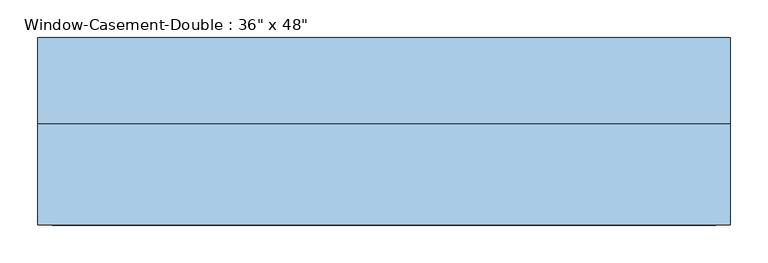
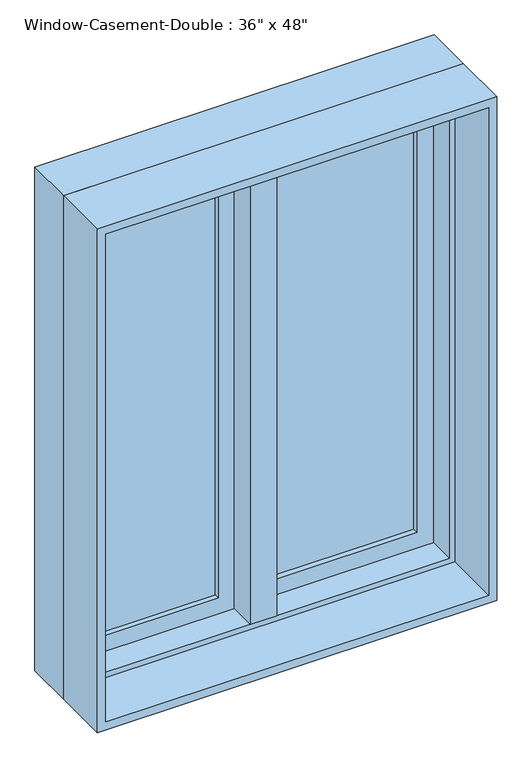
"""IFC4 building model written with IfcOpenShell, lengths in millimetres: window geometry."""

from ifc_helpers import new_model, si_unit, frame, origin, place, context, project, spatial, polyline, outline, extrude, faceted_brep, source, transform, mapped, element, save


def window_d341e8ac(model_context):
    return source(origin(), model_context, "Body", "SolidModel", [
        faceted_brep([(9.525, 133.35, 2120.9), (-9.525, 133.35, 2120.9), (-9.525, 82.55, 2120.9), (9.525, 82.55, 2120.9), (9.525, 133.35, 927.1), (9.525, 82.55, 927.1), (-9.525, 82.55, 927.1), (-9.525, 133.35, 927.1), (-9.525, 82.55, 946.15), (-9.525, 82.55, 2101.85), (-30.1625, 82.55, 946.15), (-30.1625, 82.55, 2101.85), (-30.1625, 19.05, 946.15), (-30.1625, 19.05, 2101.85), (30.1625, 19.05, 946.15), (30.1625, 19.05, 2101.85), (30.1625, 82.55, 946.15), (30.1625, 82.55, 2101.85), (9.525, 82.55, 946.15), (9.525, 82.55, 2101.85)], [[[0, 1, 2, 3]], [[4, 5, 6, 7]], [[1, 0, 4, 7]], [[2, 1, 7, 6, 8, 9]], [[9, 8, 10, 11]], [[11, 10, 12, 13]], [[13, 12, 14, 15]], [[15, 14, 16, 17]], [[17, 16, 18, 19]], [[0, 3, 19, 18, 5, 4]], [[18, 8, 6, 5]], [[9, 19, 3, 2]], [[8, 18, 16, 14, 12, 10]], [[19, 9, 11, 13, 15, 17]]]),
        extrude(outline(polyline([(-66.675, 114.3), (-66.675, 107.95), (-387.35, 107.95), (-387.35, 114.3), (-66.675, 114.3)])), frame((0.0, 0.0, 984.25), z_axis=(0.0, 0.0, 1.0), x_axis=(1.0, 0.0, 0.0)), (0.0, 0.0, 1.0), 1079.5),
        extrude(outline(polyline([(-387.35, 95.25), (-387.35, 101.6), (-66.675, 101.6), (-66.675, 95.25), (-387.35, 95.25)])), frame((0.0, 0.0, 984.25), z_axis=(0.0, 0.0, 1.0), x_axis=(1.0, 0.0, 0.0)), (0.0, 0.0, 1.0), 1079.5),
        extrude(outline(polyline([(387.35, 114.3), (387.35, 107.95), (66.675, 107.95), (66.675, 114.3), (387.35, 114.3)])), frame((0.0, 0.0, 984.25), z_axis=(0.0, 0.0, 1.0), x_axis=(1.0, 0.0, 0.0)), (0.0, 0.0, 1.0), 1079.5),
        extrude(outline(polyline([(66.675, 95.25), (66.675, 101.6), (387.35, 101.6), (387.35, 95.25), (66.675, 95.25)])), frame((0.0, 0.0, 984.25), z_axis=(0.0, 0.0, 1.0), x_axis=(1.0, 0.0, 0.0)), (0.0, 0.0, 1.0), 1079.5),
        extrude(outline(polyline([(2120.9, -444.5), (927.1, -444.5), (927.1, -9.525), (2120.9, -9.525), (2120.9, -444.5)]), holes=[polyline([(2063.75, -66.675), (984.25, -66.675), (984.25, -387.35), (2063.75, -387.35), (2063.75, -66.675)])]), frame((0.0, 82.55, 0.0), z_axis=(0.0, 1.0, 0.0), x_axis=(0.0, 0.0, 1.0)), (0.0, 0.0, 1.0), 44.45),
        extrude(outline(polyline([(927.1, 444.5), (2120.9, 444.5), (2120.9, 9.525), (927.1, 9.525), (927.1, 444.5)]), holes=[polyline([(984.25, 66.675), (2063.75, 66.675), (2063.75, 387.35), (984.25, 387.35), (984.25, 66.675)])]), frame((0.0, 82.55, 0.0), z_axis=(0.0, 1.0, 0.0), x_axis=(0.0, 0.0, 1.0)), (0.0, 0.0, 1.0), 44.45),
        extrude(outline(polyline([(2133.6, -457.2), (914.4, -457.2), (914.4, 457.2), (2133.6, 457.2), (2133.6, -457.2)]), holes=[polyline([(2114.55, 438.15), (933.45, 438.15), (933.45, -438.15), (2114.55, -438.15), (2114.55, 438.15)])]), frame((0.0, -114.3, 0.0), z_axis=(0.0, 1.0, 0.0), x_axis=(0.0, 0.0, 1.0)), (0.0, 0.0, 1.0), 133.35),
        faceted_brep([(425.45, 82.55, 2101.85), (425.45, 19.05, 2101.85), (-425.45, 19.05, 2101.85), (-425.45, 82.55, 2101.85), (444.5, 133.35, 2120.9), (444.5, 82.55, 2120.9), (-444.5, 82.55, 2120.9), (-444.5, 133.35, 2120.9), (457.2, 19.05, 2133.6), (457.2, 133.35, 2133.6), (-457.2, 133.35, 2133.6), (-457.2, 19.05, 2133.6), (-425.45, 19.05, 946.15), (-425.45, 82.55, 946.15), (-444.5, 82.55, 927.1), (-444.5, 133.35, 927.1), (-457.2, 133.35, 914.4), (-457.2, 19.05, 914.4), (425.45, 19.05, 946.15), (425.45, 82.55, 946.15), (444.5, 82.55, 927.1), (444.5, 133.35, 927.1), (457.2, 133.35, 914.4), (457.2, 19.05, 914.4)], [[[0, 1, 2, 3]], [[4, 5, 6, 7]], [[8, 9, 10, 11]], [[3, 2, 12, 13]], [[7, 6, 14, 15]], [[11, 10, 16, 17]], [[13, 12, 18, 19]], [[15, 14, 20, 21]], [[17, 16, 22, 23]], [[11, 17, 23, 8], [1, 18, 12, 2]], [[19, 18, 1, 0]], [[5, 20, 14, 6], [3, 13, 19, 0]], [[21, 20, 5, 4]], [[23, 22, 9, 8]], [[9, 22, 16, 10], [7, 15, 21, 4]]]),
    ])


if __name__ == "__main__":
    model = new_model("IFC4")
    model_context = context("Model", 3, world=origin())
    ifc_project = project(units=[si_unit("LENGTHUNIT", "METRE", prefix="MILLI")], contexts=[model_context])
    site = spatial("IfcSite", under=ifc_project)
    building = spatial("IfcBuilding", under=site)
    placement = place(None, origin())
    window_shape = window_d341e8ac(model_context)
    element("IfcWindow", 1, ObjectType="Window-Casement-Double : 36\" x 48\"", at=placement, inside=building, context=model_context, shape_type="MappedRepresentation", body=[
        mapped(window_shape, transform((0.0, 0.0, 0.0), x_axis=(1.0, 0.0, 0.0), y_axis=(0.0, 1.0, 0.0), z_axis=(0.0, 0.0, 1.0))),
    ])
    save(model, "model.ifc")

# Revit data of these elements
# Type "Window-Casement-Double : 36\" x 48\""
#   Type Mark = "14"
#   Fire Rating = "0.5h"
#   Assembly Code = "B2020100"
#   Analytic Construction = "Double glazing - domestic"
#   Frame Extension [instance default] = 0' - 0 1/4"
#   Window Inset [instance default] = 0' - 0"
#   Wall Thickness [instance default] = 0' - 6"
#   Interior Wall Closure [instance default] = 0' - 2 1/4"
#   Half Width = 1' - 6"
#   Visual Light Transmittance = 0.81
#   Thermal Resistance (R) = 1.8146 (h·ft²·°F)/BTU
#   Solar Heat Gain Coefficient = 0.76
#   Rough Width = 3' - 0 1/2"
#   Rough Height = 4' - 0 1/2"
#   Height = 4' - 0"
#   Heat Transfer Coefficient (U) = 0.5511 BTU/(h·ft²·°F)
#   Exterior Wall Closure [instance default] = 0' - 1 1/4"
#   Extension Jamb [instance default] = 0' - 2 1/4"
#   Default Sill Height = 3' - 0"
#   Width = 3' - 0"
#   Define Thermal Properties by = 0
#   Muntin Visibility = yes
#   Interior Trim Visibility [instance default] = yes
#   Exterior Trim Visibility [instance default] = yes
#   Extension Jamb Visibility [instance default] = yes
#   Interior Trim Material = Wood - Stained
#   Muntin Pattern = Muntin Pattern_2x2 : Muntin Pattern_2x2
#   Interior Trim = Trim-Window-Interior-Flat : Picture Frame
#   Interior Frame Material = Wood - Stained
#   Glass Panel Material = Glass
#   Exterior Trim Material = Clad - White
#   Exterior Trim = Trim-Window-Exterior-Flat : with Sill
#   Exterior Frame Material = Clad - White
#   Wall Closure = (empty or 0)
# Element 1 (IfcWindow, "Window-Casement-Double : 36\" x 48\"")
#   Wall Thickness = 0' - 9"
#   Extension Jamb = 0' - 5 1/4"
#   Materials on its faces: "Wood - Stained", "Glass", "Clad - White"
# Materials
#   "Wood - Stained": class "Wood", colour RGB 224 178 126, transparency 0, Cost = 0
#   "Glass": class "Glass", colour RGB 0 128 192, transparency 0.75, Description = "Soda Lime Glass", Cost = 0
#   "Clad - White": class "Wood", colour RGB 242 242 238, transparency 0, Cost = 0
